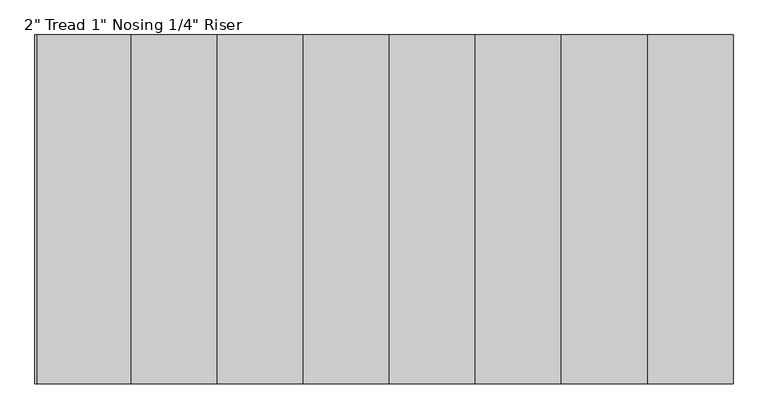
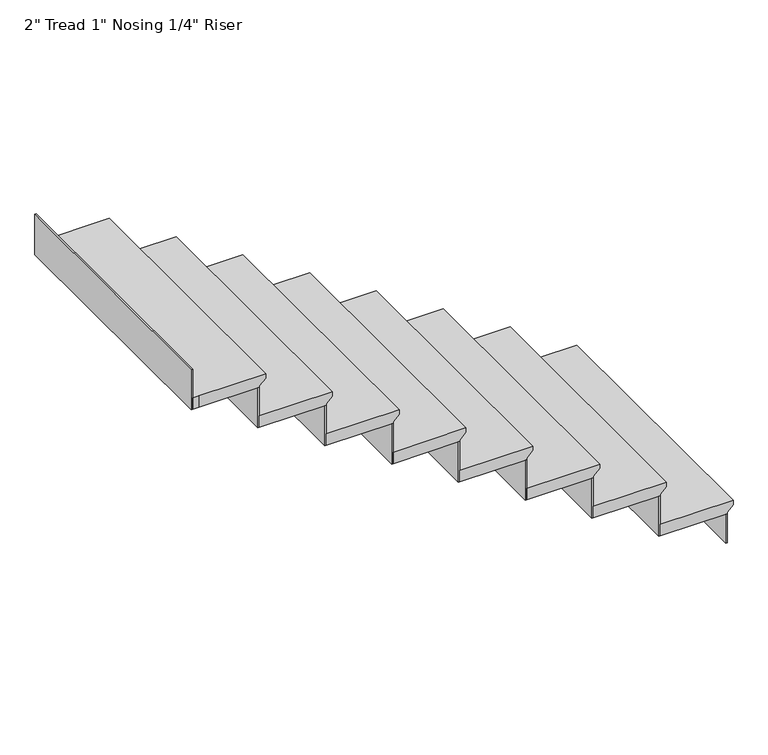
"""IFC4 building model written with IfcOpenShell, lengths in millimetres: stair flight geometry."""

from ifc_helpers import new_model, si_unit, origin, place, context, project, spatial, faceted_brep, source, transform, mapped, element, save


def stair_flight_3c50d200(model_context):
    return source(origin(), model_context, "Body", "Brep", [
        faceted_brep([(-7986.2683044, -2706.1923176, 3359.15), (-7986.2683044, -2706.1923176, 3378.2), (-7986.2683044, -3838.3891189, 3378.2), (-7986.2683044, -3838.3891189, 3359.15), (-8011.6683044, -2706.1923176, 3333.75), (-8011.6683044, -3838.3891189, 3333.75), (-8291.0683044, -2706.1923176, 3378.2), (-8291.0683044, -3838.3891189, 3378.2), (-8011.6683044, -3838.3891189, 3327.4), (-8291.0683044, -3838.3891189, 3327.4), (-8291.0683044, -2706.1923176, 3327.4), (-8011.6683044, -2706.1923176, 3327.4)], [[[0, 1, 2, 3]], [[4, 0, 3, 5]], [[2, 1, 6, 7]], [[8, 9, 10, 11]], [[2, 7, 9, 8, 5, 3]], [[8, 11, 4, 5]], [[6, 1, 0, 4, 11, 10]], [[7, 6, 10, 9]]]),
        faceted_brep([(-8011.6683044, -2706.1923176, 3327.4), (-8011.6683044, -2706.1923176, 3200.4), (-8018.0183044, -2706.1923176, 3200.4), (-8018.0183044, -2706.1923176, 3327.4), (-8011.6683044, -3838.3891189, 3327.4), (-8018.0183044, -3838.3891189, 3327.4), (-8018.0183044, -3838.3891189, 3200.4), (-8011.6683044, -3838.3891189, 3200.4)], [[[0, 1, 2, 3]], [[4, 5, 6, 7]], [[1, 0, 4, 7]], [[2, 1, 7, 6]], [[3, 2, 6, 5]], [[0, 3, 5, 4]]]),
        faceted_brep([(-8291.0683044, -2706.1923176, 3505.2), (-8291.0683044, -2706.1923176, 3327.4), (-8297.4183044, -2706.1923176, 3327.4), (-8297.4183044, -2706.1923176, 3505.2), (-8291.0683044, -3838.3891189, 3505.2), (-8297.4183044, -3838.3891189, 3505.2), (-8297.4183044, -3838.3891189, 3327.4), (-8291.0683044, -3838.3891189, 3327.4)], [[[0, 1, 2, 3]], [[4, 5, 6, 7]], [[1, 0, 4, 7]], [[2, 1, 7, 6]], [[3, 2, 6, 5]], [[0, 3, 5, 4]]]),
        faceted_brep([(-8265.6683044, -3838.3891189, 3556.0), (-8265.6683044, -2706.1923176, 3556.0), (-8570.4683044, -2706.1923176, 3556.0), (-8570.4683044, -3838.3891189, 3556.0), (-8291.0683044, -3838.3891189, 3505.2), (-8570.4683044, -3838.3891189, 3505.2), (-8570.4683044, -2706.1923176, 3505.2), (-8291.0683044, -2706.1923176, 3505.2), (-8291.0683044, -3838.3891189, 3511.55), (-8265.6683044, -3838.3891189, 3536.95), (-8291.0683044, -2706.1923176, 3511.55), (-8265.6683044, -2706.1923176, 3536.95)], [[[0, 1, 2, 3]], [[4, 5, 6, 7]], [[0, 3, 5, 4, 8, 9]], [[4, 7, 10, 8]], [[2, 1, 11, 10, 7, 6]], [[3, 2, 6, 5]], [[11, 1, 0, 9]], [[10, 11, 9, 8]]]),
        faceted_brep([(-8570.4683044, -2706.1923176, 3683.0), (-8570.4683044, -2706.1923176, 3505.2), (-8576.8183044, -2706.1923176, 3505.2), (-8576.8183044, -2706.1923176, 3683.0), (-8570.4683044, -3838.3891189, 3683.0), (-8576.8183044, -3838.3891189, 3683.0), (-8576.8183044, -3838.3891189, 3505.2), (-8570.4683044, -3838.3891189, 3505.2)], [[[0, 1, 2, 3]], [[4, 5, 6, 7]], [[1, 0, 4, 7]], [[2, 1, 7, 6]], [[3, 2, 6, 5]], [[0, 3, 5, 4]]]),
        faceted_brep([(-8545.0683044, -3838.3891189, 3733.8), (-8545.0683044, -2706.1923176, 3733.8), (-8849.8683044, -2706.1923176, 3733.8), (-8849.8683044, -3838.3891189, 3733.8), (-8570.4683044, -3838.3891189, 3683.0), (-8849.8683044, -3838.3891189, 3683.0), (-8849.8683044, -2706.1923176, 3683.0), (-8570.4683044, -2706.1923176, 3683.0), (-8570.4683044, -3838.3891189, 3689.35), (-8545.0683044, -3838.3891189, 3714.75), (-8570.4683044, -2706.1923176, 3689.35), (-8545.0683044, -2706.1923176, 3714.75)], [[[0, 1, 2, 3]], [[4, 5, 6, 7]], [[0, 3, 5, 4, 8, 9]], [[4, 7, 10, 8]], [[2, 1, 11, 10, 7, 6]], [[3, 2, 6, 5]], [[11, 1, 0, 9]], [[10, 11, 9, 8]]]),
        faceted_brep([(-8849.8683044, -2706.1923176, 3860.8), (-8849.8683044, -2706.1923176, 3683.0), (-8856.2183044, -2706.1923176, 3683.0), (-8856.2183044, -2706.1923176, 3860.8), (-8849.8683044, -3838.3891189, 3860.8), (-8856.2183044, -3838.3891189, 3860.8), (-8856.2183044, -3838.3891189, 3683.0), (-8849.8683044, -3838.3891189, 3683.0)], [[[0, 1, 2, 3]], [[4, 5, 6, 7]], [[1, 0, 4, 7]], [[2, 1, 7, 6]], [[3, 2, 6, 5]], [[0, 3, 5, 4]]]),
        faceted_brep([(-8824.4683044, -3838.3891189, 3911.6), (-8824.4683044, -2706.1923176, 3911.6), (-9129.2683044, -2706.1923176, 3911.6), (-9129.2683044, -3838.3891189, 3911.6), (-8849.8683044, -3838.3891189, 3860.8), (-9129.2683044, -3838.3891189, 3860.8), (-9129.2683044, -2706.1923176, 3860.8), (-8849.8683044, -2706.1923176, 3860.8), (-8849.8683044, -3838.3891189, 3867.15), (-8824.4683044, -3838.3891189, 3892.55), (-8849.8683044, -2706.1923176, 3867.15), (-8824.4683044, -2706.1923176, 3892.55)], [[[0, 1, 2, 3]], [[4, 5, 6, 7]], [[0, 3, 5, 4, 8, 9]], [[4, 7, 10, 8]], [[2, 1, 11, 10, 7, 6]], [[3, 2, 6, 5]], [[11, 1, 0, 9]], [[10, 11, 9, 8]]]),
        faceted_brep([(-9129.2683044, -2706.1923176, 4038.6), (-9129.2683044, -2706.1923176, 3860.8), (-9135.6183044, -2706.1923176, 3860.8), (-9135.6183044, -2706.1923176, 4038.6), (-9129.2683044, -3838.3891189, 4038.6), (-9135.6183044, -3838.3891189, 4038.6), (-9135.6183044, -3838.3891189, 3860.8), (-9129.2683044, -3838.3891189, 3860.8)], [[[0, 1, 2, 3]], [[4, 5, 6, 7]], [[1, 0, 4, 7]], [[2, 1, 7, 6]], [[3, 2, 6, 5]], [[0, 3, 5, 4]]]),
        faceted_brep([(-9103.8683044, -3838.3891189, 4089.4), (-9103.8683044, -2706.1923176, 4089.4), (-9408.6683044, -2706.1923176, 4089.4), (-9408.6683044, -3838.3891189, 4089.4), (-9129.2683044, -3838.3891189, 4038.6), (-9408.6683044, -3838.3891189, 4038.6), (-9408.6683044, -2706.1923176, 4038.6), (-9129.2683044, -2706.1923176, 4038.6), (-9129.2683044, -3838.3891189, 4044.95), (-9103.8683044, -3838.3891189, 4070.35), (-9129.2683044, -2706.1923176, 4044.95), (-9103.8683044, -2706.1923176, 4070.35)], [[[0, 1, 2, 3]], [[4, 5, 6, 7]], [[0, 3, 5, 4, 8, 9]], [[4, 7, 10, 8]], [[2, 1, 11, 10, 7, 6]], [[3, 2, 6, 5]], [[11, 1, 0, 9]], [[10, 11, 9, 8]]]),
        faceted_brep([(-9408.6683044, -2706.1923176, 4216.4), (-9408.6683044, -2706.1923176, 4038.6), (-9415.0183044, -2706.1923176, 4038.6), (-9415.0183044, -2706.1923176, 4216.4), (-9408.6683044, -3838.3891189, 4216.4), (-9415.0183044, -3838.3891189, 4216.4), (-9415.0183044, -3838.3891189, 4038.6), (-9408.6683044, -3838.3891189, 4038.6)], [[[0, 1, 2, 3]], [[4, 5, 6, 7]], [[1, 0, 4, 7]], [[2, 1, 7, 6]], [[3, 2, 6, 5]], [[0, 3, 5, 4]]]),
        faceted_brep([(-9383.2683044, -3838.3891189, 4267.2), (-9383.2683044, -2706.1923176, 4267.2), (-9688.0683044, -2706.1923176, 4267.2), (-9688.0683044, -3838.3891189, 4267.2), (-9408.6683044, -3838.3891189, 4216.4), (-9688.0683044, -3838.3891189, 4216.4), (-9688.0683044, -2706.1923176, 4216.4), (-9408.6683044, -2706.1923176, 4216.4), (-9408.6683044, -3838.3891189, 4222.75), (-9383.2683044, -3838.3891189, 4248.15), (-9408.6683044, -2706.1923176, 4222.75), (-9383.2683044, -2706.1923176, 4248.15)], [[[0, 1, 2, 3]], [[4, 5, 6, 7]], [[0, 3, 5, 4, 8, 9]], [[4, 7, 10, 8]], [[2, 1, 11, 10, 7, 6]], [[3, 2, 6, 5]], [[11, 1, 0, 9]], [[10, 11, 9, 8]]]),
        faceted_brep([(-9688.0683044, -2706.1923176, 4394.2), (-9688.0683044, -2706.1923176, 4216.4), (-9694.4183044, -2706.1923176, 4216.4), (-9694.4183044, -2706.1923176, 4394.2), (-9688.0683044, -3838.3891189, 4394.2), (-9694.4183044, -3838.3891189, 4394.2), (-9694.4183044, -3838.3891189, 4216.4), (-9688.0683044, -3838.3891189, 4216.4)], [[[0, 1, 2, 3]], [[4, 5, 6, 7]], [[1, 0, 4, 7]], [[2, 1, 7, 6]], [[3, 2, 6, 5]], [[0, 3, 5, 4]]]),
        faceted_brep([(-9662.6683044, -3838.3891189, 4445.0), (-9662.6683044, -2706.1923176, 4445.0), (-9967.4683044, -2706.1923176, 4445.0), (-9967.4683044, -3838.3891189, 4445.0), (-9688.0683044, -3838.3891189, 4394.2), (-9967.4683044, -3838.3891189, 4394.2), (-9967.4683044, -2706.1923176, 4394.2), (-9688.0683044, -2706.1923176, 4394.2), (-9688.0683044, -3838.3891189, 4400.55), (-9662.6683044, -3838.3891189, 4425.95), (-9688.0683044, -2706.1923176, 4400.55), (-9662.6683044, -2706.1923176, 4425.95)], [[[0, 1, 2, 3]], [[4, 5, 6, 7]], [[0, 3, 5, 4, 8, 9]], [[4, 7, 10, 8]], [[2, 1, 11, 10, 7, 6]], [[3, 2, 6, 5]], [[11, 1, 0, 9]], [[10, 11, 9, 8]]]),
        faceted_brep([(-10246.8683044, -2706.1923176, 4749.8), (-10246.8683044, -2706.1923176, 4572.0), (-10253.2183044, -2706.1923176, 4572.0), (-10253.2183044, -2706.1923176, 4749.8), (-10246.8683044, -3838.3891189, 4749.8), (-10253.2183044, -3838.3891189, 4749.8), (-10253.2183044, -3838.3891189, 4572.0), (-10246.8683044, -3838.3891189, 4572.0)], [[[0, 1, 2, 3]], [[4, 5, 6, 7]], [[1, 0, 4, 7]], [[2, 1, 7, 6]], [[3, 2, 6, 5]], [[0, 3, 5, 4]]]),
        faceted_brep([(-9967.4683044, -2706.1923176, 4572.0), (-9967.4683044, -2706.1923176, 4394.2), (-9973.8183044, -2706.1923176, 4394.2), (-9973.8183044, -2706.1923176, 4572.0), (-9967.4683044, -3838.3891189, 4572.0), (-9973.8183044, -3838.3891189, 4572.0), (-9973.8183044, -3838.3891189, 4394.2), (-9967.4683044, -3838.3891189, 4394.2)], [[[0, 1, 2, 3]], [[4, 5, 6, 7]], [[1, 0, 4, 7]], [[2, 1, 7, 6]], [[3, 2, 6, 5]], [[0, 3, 5, 4]]]),
        faceted_brep([(-10246.8683044, -3838.3891189, 4622.8), (-10221.4683044, -3838.3891189, 4622.8), (-9942.0683044, -3838.3891189, 4622.8), (-9942.0683044, -2706.1923176, 4622.8), (-10246.8683044, -2706.1923176, 4622.8), (-10221.4683044, -3838.3891189, 4572.0), (-10246.8683044, -3838.3891189, 4572.0), (-10246.8683044, -2706.1923176, 4572.0), (-9967.4683044, -2706.1923176, 4572.0), (-9967.4683044, -3838.3891189, 4572.0), (-9967.4683044, -3838.3891189, 4578.35), (-9942.0683044, -3838.3891189, 4603.75), (-9967.4683044, -2706.1923176, 4578.35), (-9942.0683044, -2706.1923176, 4603.75)], [[[0, 1, 2, 3, 4]], [[5, 6, 7, 8, 9]], [[1, 0, 6, 5]], [[2, 1, 5, 9, 10, 11]], [[9, 8, 12, 10]], [[4, 3, 13, 12, 8, 7]], [[0, 4, 7, 6]], [[13, 3, 2, 11]], [[12, 13, 11, 10]]]),
    ])


if __name__ == "__main__":
    model = new_model("IFC4")
    model_context = context("Model", 3, world=origin())
    ifc_project = project(units=[si_unit("LENGTHUNIT", "METRE", prefix="MILLI")], contexts=[model_context])
    site = spatial("IfcSite", under=ifc_project)
    building = spatial("IfcBuilding", under=site)
    placement = place(None, origin())
    stair_flight_shape = stair_flight_3c50d200(model_context)
    element("IfcStairFlight", 1, ObjectType="2\" Tread 1\" Nosing 1/4\" Riser", at=placement, inside=building, context=model_context, shape_type="MappedRepresentation", body=[
        mapped(stair_flight_shape, transform((0.0, 0.0, 0.0), x_axis=(1.0, 0.0, 0.0), y_axis=(0.0, 1.0, 0.0), z_axis=(0.0, 0.0, 1.0))),
    ])
    save(model, "model.ifc")
